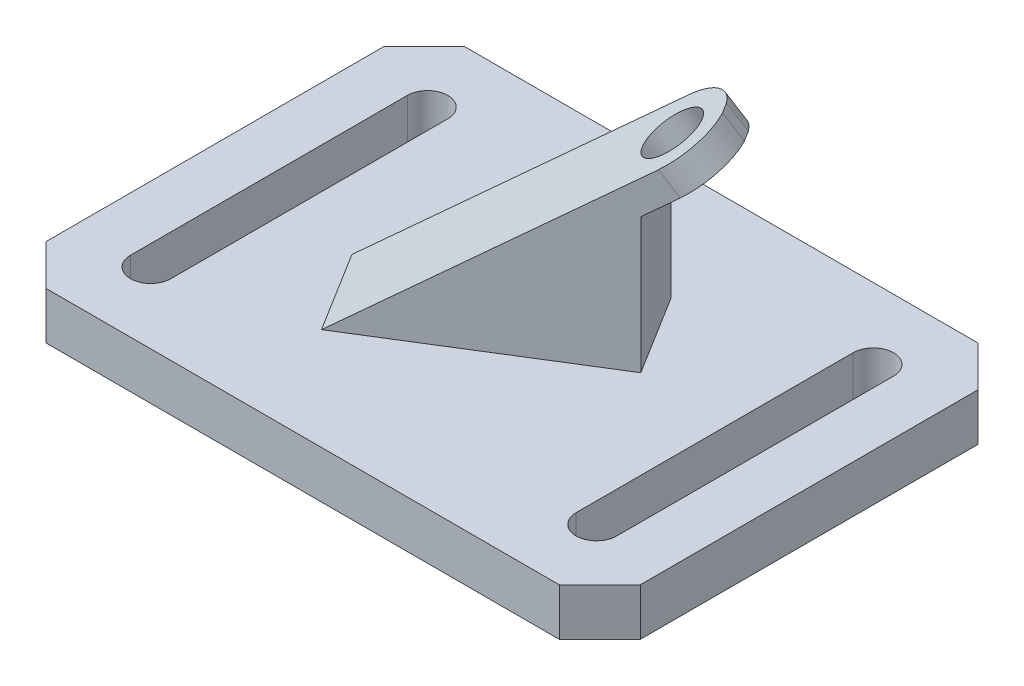
ISO-10303-21;
HEADER;
FILE_DESCRIPTION(('STEP AP214'),'2;1');
FILE_NAME('part.step','',(''),(''),'','','');
FILE_SCHEMA(('AUTOMOTIVE_DESIGN { 1 0 10303 214 1 1 1 1 }'));
ENDSEC;
DATA;
#1=APPLICATION_CONTEXT('core data for automotive mechanical design processes');
#2=APPLICATION_PROTOCOL_DEFINITION('international standard','automotive_design',2000,#1);
#3=PRODUCT_CONTEXT('',#1,'mechanical');
#4=PRODUCT('Part','Part','',(#3));
#5=PRODUCT_RELATED_PRODUCT_CATEGORY('part','',(#4));
#6=PRODUCT_DEFINITION_FORMATION('','',#4);
#7=PRODUCT_DEFINITION_CONTEXT('part definition',#1,'design');
#8=PRODUCT_DEFINITION('design','',#6,#7);
#9=PRODUCT_DEFINITION_SHAPE('','',#8);
#10=(LENGTH_UNIT() NAMED_UNIT(*) SI_UNIT(.MILLI.,.METRE.));
#11=(NAMED_UNIT(*) PLANE_ANGLE_UNIT() SI_UNIT($,.RADIAN.));
#12=(NAMED_UNIT(*) SI_UNIT($,.STERADIAN.) SOLID_ANGLE_UNIT());
#13=UNCERTAINTY_MEASURE_WITH_UNIT(LENGTH_MEASURE(1.E-05),#10,'distance_accuracy_value','');
#14=(GEOMETRIC_REPRESENTATION_CONTEXT(3) GLOBAL_UNCERTAINTY_ASSIGNED_CONTEXT((#13)) GLOBAL_UNIT_ASSIGNED_CONTEXT((#10,
#11,#12)) REPRESENTATION_CONTEXT('',''));
#15=CARTESIAN_POINT('',(0.,0.,0.));
#16=DIRECTION('',(0.,0.,1.));
#17=DIRECTION('',(1.,0.,0.));
#18=AXIS2_PLACEMENT_3D('',#15,#16,#17);
#19=CARTESIAN_POINT('',(0.,7.,0.));
#20=DIRECTION('',(0.,-1.,0.));
#21=DIRECTION('',(0.,0.,-1.));
#22=AXIS2_PLACEMENT_3D('',#19,#20,#21);
#23=PLANE('',#22);
#24=DIRECTION('',(-1.,0.,0.));
#25=VECTOR('',#24,1.);
#26=CARTESIAN_POINT('',(-44.,7.,-31.));
#27=LINE('',#26,#25);
#28=CARTESIAN_POINT('',(38.,7.,-31.));
#29=VERTEX_POINT('',#28);
#30=CARTESIAN_POINT('',(-38.,7.,-31.));
#31=VERTEX_POINT('',#30);
#32=EDGE_CURVE('E330',#29,#31,#27,.T.);
#33=ORIENTED_EDGE('',*,*,#32,.T.);
#34=DIRECTION('',(0.707106781186548,0.,-0.707106781186547));
#35=VECTOR('',#34,1.);
#36=CARTESIAN_POINT('',(-44.,7.,-25.));
#37=LINE('',#36,#35);
#38=CARTESIAN_POINT('',(-44.,7.,-25.));
#39=VERTEX_POINT('',#38);
#40=EDGE_CURVE('E372',#31,#39,#37,.F.);
#41=ORIENTED_EDGE('',*,*,#40,.T.);
#42=DIRECTION('',(0.,0.,1.));
#43=VECTOR('',#42,1.);
#44=CARTESIAN_POINT('',(-44.,7.,31.));
#45=LINE('',#44,#43);
#46=CARTESIAN_POINT('',(-44.,7.,25.));
#47=VERTEX_POINT('',#46);
#48=EDGE_CURVE('E333',#39,#47,#45,.T.);
#49=ORIENTED_EDGE('',*,*,#48,.T.);
#50=DIRECTION('',(-0.707106781186547,0.,-0.707106781186548));
#51=VECTOR('',#50,1.);
#52=CARTESIAN_POINT('',(-38.,7.,31.));
#53=LINE('',#52,#51);
#54=CARTESIAN_POINT('',(-38.,7.,31.));
#55=VERTEX_POINT('',#54);
#56=EDGE_CURVE('E368',#47,#55,#53,.F.);
#57=ORIENTED_EDGE('',*,*,#56,.T.);
#58=DIRECTION('',(1.,0.,0.));
#59=VECTOR('',#58,1.);
#60=CARTESIAN_POINT('',(-44.,7.,31.));
#61=LINE('',#60,#59);
#62=CARTESIAN_POINT('',(38.,7.,31.));
#63=VERTEX_POINT('',#62);
#64=EDGE_CURVE('E337',#55,#63,#61,.T.);
#65=ORIENTED_EDGE('',*,*,#64,.T.);
#66=DIRECTION('',(-0.707106781186548,0.,0.707106781186547));
#67=VECTOR('',#66,1.);
#68=CARTESIAN_POINT('',(44.,7.,25.));
#69=LINE('',#68,#67);
#70=CARTESIAN_POINT('',(44.,7.,25.));
#71=VERTEX_POINT('',#70);
#72=EDGE_CURVE('E369',#63,#71,#69,.F.);
#73=ORIENTED_EDGE('',*,*,#72,.T.);
#74=DIRECTION('',(0.,0.,-1.));
#75=VECTOR('',#74,1.);
#76=CARTESIAN_POINT('',(44.,7.,31.));
#77=LINE('',#76,#75);
#78=CARTESIAN_POINT('',(44.,7.,-25.));
#79=VERTEX_POINT('',#78);
#80=EDGE_CURVE('E329',#71,#79,#77,.T.);
#81=ORIENTED_EDGE('',*,*,#80,.T.);
#82=DIRECTION('',(0.707106781186547,0.,0.707106781186548));
#83=VECTOR('',#82,1.);
#84=CARTESIAN_POINT('',(38.,7.,-31.));
#85=LINE('',#84,#83);
#86=EDGE_CURVE('E375',#79,#29,#85,.F.);
#87=ORIENTED_EDGE('',*,*,#86,.T.);
#88=EDGE_LOOP('',(#33,#41,#49,#57,#65,#73,#81,#87));
#89=FACE_BOUND('',#88,.T.);
#90=DIRECTION('',(0.,0.,1.));
#91=VECTOR('',#90,1.);
#92=CARTESIAN_POINT('',(-36.,7.,-20.5));
#93=LINE('',#92,#91);
#94=CARTESIAN_POINT('',(-36.,7.,-20.5));
#95=VERTEX_POINT('',#94);
#96=CARTESIAN_POINT('',(-36.,7.,20.5));
#97=VERTEX_POINT('',#96);
#98=EDGE_CURVE('E299',#95,#97,#93,.T.);
#99=ORIENTED_EDGE('',*,*,#98,.F.);
#100=CARTESIAN_POINT('',(-33.,7.,-20.5));
#101=DIRECTION('',(0.,1.,0.));
#102=DIRECTION('',(0.,0.,1.));
#103=AXIS2_PLACEMENT_3D('',#100,#101,#102);
#104=CIRCLE('',#103,3.);
#105=CARTESIAN_POINT('',(-30.,7.,-20.5));
#106=VERTEX_POINT('',#105);
#107=EDGE_CURVE('E300',#106,#95,#104,.T.);
#108=ORIENTED_EDGE('',*,*,#107,.F.);
#109=DIRECTION('',(0.,0.,-1.));
#110=VECTOR('',#109,1.);
#111=CARTESIAN_POINT('',(-30.,7.,-20.5));
#112=LINE('',#111,#110);
#113=CARTESIAN_POINT('',(-30.,7.,20.5));
#114=VERTEX_POINT('',#113);
#115=EDGE_CURVE('E304',#114,#106,#112,.T.);
#116=ORIENTED_EDGE('',*,*,#115,.F.);
#117=CARTESIAN_POINT('',(-33.,7.,20.5));
#118=DIRECTION('',(0.,1.,0.));
#119=DIRECTION('',(0.,0.,1.));
#120=AXIS2_PLACEMENT_3D('',#117,#118,#119);
#121=CIRCLE('',#120,3.);
#122=EDGE_CURVE('E305',#97,#114,#121,.T.);
#123=ORIENTED_EDGE('',*,*,#122,.F.);
#124=EDGE_LOOP('',(#99,#108,#116,#123));
#125=FACE_BOUND('',#124,.T.);
#126=DIRECTION('',(-0.849441251034907,0.,0.527683201400473));
#127=VECTOR('',#126,1.);
#128=CARTESIAN_POINT('',(42.4093895965386,7.,-34.5859380339113));
#129=LINE('',#128,#127);
#130=CARTESIAN_POINT('',(9.45877731415572,7.,-14.116618282734));
#131=VERTEX_POINT('',#130);
#132=CARTESIAN_POINT('',(-19.7049573891051,7.,4.00024721474623));
#133=VERTEX_POINT('',#132);
#134=EDGE_CURVE('E259',#131,#133,#129,.T.);
#135=ORIENTED_EDGE('',*,*,#134,.F.);
#136=DIRECTION('',(0.527683201400473,0.,0.849441251034907));
#137=VECTOR('',#136,1.);
#138=CARTESIAN_POINT('',(-29.0620963880788,7.,-76.1258296082822));
#139=LINE('',#138,#137);
#140=CARTESIAN_POINT('',(16.8463421337624,7.,-2.22444076824528));
#141=VERTEX_POINT('',#140);
#142=EDGE_CURVE('E245',#131,#141,#139,.T.);
#143=ORIENTED_EDGE('',*,*,#142,.T.);
#144=DIRECTION('',(0.849441251034907,0.,-0.527683201400473));
#145=VECTOR('',#144,1.);
#146=CARTESIAN_POINT('',(-12.3173925694985,7.,15.892424729235));
#147=LINE('',#146,#145);
#148=CARTESIAN_POINT('',(-12.3173925694985,7.,15.892424729235));
#149=VERTEX_POINT('',#148);
#150=EDGE_CURVE('E262',#149,#141,#147,.T.);
#151=ORIENTED_EDGE('',*,*,#150,.F.);
#152=DIRECTION('',(0.527683201400473,0.,0.849441251034907));
#153=VECTOR('',#152,1.);
#154=CARTESIAN_POINT('',(-19.7049573891051,7.,4.00024721474623));
#155=LINE('',#154,#153);
#156=EDGE_CURVE('E227',#133,#149,#155,.T.);
#157=ORIENTED_EDGE('',*,*,#156,.F.);
#158=EDGE_LOOP('',(#135,#143,#151,#157));
#159=FACE_BOUND('',#158,.T.);
#160=CARTESIAN_POINT('',(33.,7.,-20.5));
#161=DIRECTION('',(0.,1.,0.));
#162=DIRECTION('',(0.,0.,1.));
#163=AXIS2_PLACEMENT_3D('',#160,#161,#162);
#164=CIRCLE('',#163,2.99999999999999);
#165=CARTESIAN_POINT('',(36.,7.,-20.5));
#166=VERTEX_POINT('',#165);
#167=CARTESIAN_POINT('',(30.,7.,-20.5));
#168=VERTEX_POINT('',#167);
#169=EDGE_CURVE('E265',#166,#168,#164,.T.);
#170=ORIENTED_EDGE('',*,*,#169,.F.);
#171=DIRECTION('',(0.,0.,-1.));
#172=VECTOR('',#171,1.);
#173=CARTESIAN_POINT('',(36.,7.,-20.5));
#174=LINE('',#173,#172);
#175=CARTESIAN_POINT('',(36.,7.,20.5));
#176=VERTEX_POINT('',#175);
#177=EDGE_CURVE('E274',#176,#166,#174,.T.);
#178=ORIENTED_EDGE('',*,*,#177,.F.);
#179=CARTESIAN_POINT('',(33.,7.,20.5));
#180=DIRECTION('',(0.,1.,0.));
#181=DIRECTION('',(0.,0.,1.));
#182=AXIS2_PLACEMENT_3D('',#179,#180,#181);
#183=CIRCLE('',#182,3.);
#184=CARTESIAN_POINT('',(30.,7.,20.5));
#185=VERTEX_POINT('',#184);
#186=EDGE_CURVE('E272',#185,#176,#183,.T.);
#187=ORIENTED_EDGE('',*,*,#186,.F.);
#188=DIRECTION('',(0.,0.,1.));
#189=VECTOR('',#188,1.);
#190=CARTESIAN_POINT('',(30.,7.,-20.5));
#191=LINE('',#190,#189);
#192=EDGE_CURVE('E268',#168,#185,#191,.T.);
#193=ORIENTED_EDGE('',*,*,#192,.F.);
#194=EDGE_LOOP('',(#170,#178,#187,#193));
#195=FACE_BOUND('',#194,.T.);
#196=ADVANCED_FACE('F41',(#89,#125,#159,#195),#23,.F.);
#197=CARTESIAN_POINT('',(0.,0.,0.));
#198=DIRECTION('',(0.,-1.,0.));
#199=DIRECTION('',(0.,0.,-1.));
#200=AXIS2_PLACEMENT_3D('',#197,#198,#199);
#201=PLANE('',#200);
#202=DIRECTION('',(0.,0.,1.));
#203=VECTOR('',#202,1.);
#204=CARTESIAN_POINT('',(-44.,0.,31.));
#205=LINE('',#204,#203);
#206=CARTESIAN_POINT('',(-44.,0.,-25.));
#207=VERTEX_POINT('',#206);
#208=CARTESIAN_POINT('',(-44.,0.,25.));
#209=VERTEX_POINT('',#208);
#210=EDGE_CURVE('E343',#207,#209,#205,.T.);
#211=ORIENTED_EDGE('',*,*,#210,.F.);
#212=DIRECTION('',(-0.707106781186548,0.,0.707106781186547));
#213=VECTOR('',#212,1.);
#214=CARTESIAN_POINT('',(-34.5,0.,-34.5));
#215=LINE('',#214,#213);
#216=CARTESIAN_POINT('',(-38.,0.,-31.));
#217=VERTEX_POINT('',#216);
#218=EDGE_CURVE('E359',#207,#217,#215,.F.);
#219=ORIENTED_EDGE('',*,*,#218,.T.);
#220=DIRECTION('',(-1.,0.,0.));
#221=VECTOR('',#220,1.);
#222=CARTESIAN_POINT('',(-44.,0.,-31.));
#223=LINE('',#222,#221);
#224=CARTESIAN_POINT('',(38.,0.,-31.));
#225=VERTEX_POINT('',#224);
#226=EDGE_CURVE('E345',#225,#217,#223,.T.);
#227=ORIENTED_EDGE('',*,*,#226,.F.);
#228=DIRECTION('',(-0.707106781186547,0.,-0.707106781186548));
#229=VECTOR('',#228,1.);
#230=CARTESIAN_POINT('',(34.5,0.,-34.5));
#231=LINE('',#230,#229);
#232=CARTESIAN_POINT('',(44.,0.,-25.));
#233=VERTEX_POINT('',#232);
#234=EDGE_CURVE('E356',#225,#233,#231,.F.);
#235=ORIENTED_EDGE('',*,*,#234,.T.);
#236=DIRECTION('',(0.,0.,-1.));
#237=VECTOR('',#236,1.);
#238=CARTESIAN_POINT('',(44.,0.,31.));
#239=LINE('',#238,#237);
#240=CARTESIAN_POINT('',(44.,0.,25.));
#241=VERTEX_POINT('',#240);
#242=EDGE_CURVE('E327',#241,#233,#239,.T.);
#243=ORIENTED_EDGE('',*,*,#242,.F.);
#244=DIRECTION('',(0.707106781186548,0.,-0.707106781186547));
#245=VECTOR('',#244,1.);
#246=CARTESIAN_POINT('',(34.5,0.,34.5));
#247=LINE('',#246,#245);
#248=CARTESIAN_POINT('',(38.,0.,31.));
#249=VERTEX_POINT('',#248);
#250=EDGE_CURVE('E358',#241,#249,#247,.F.);
#251=ORIENTED_EDGE('',*,*,#250,.T.);
#252=DIRECTION('',(1.,0.,0.));
#253=VECTOR('',#252,1.);
#254=CARTESIAN_POINT('',(-44.,0.,31.));
#255=LINE('',#254,#253);
#256=CARTESIAN_POINT('',(-38.,0.,31.));
#257=VERTEX_POINT('',#256);
#258=EDGE_CURVE('E331',#257,#249,#255,.T.);
#259=ORIENTED_EDGE('',*,*,#258,.F.);
#260=DIRECTION('',(0.707106781186547,0.,0.707106781186548));
#261=VECTOR('',#260,1.);
#262=CARTESIAN_POINT('',(-34.5,0.,34.5));
#263=LINE('',#262,#261);
#264=EDGE_CURVE('E352',#257,#209,#263,.F.);
#265=ORIENTED_EDGE('',*,*,#264,.T.);
#266=EDGE_LOOP('',(#211,#219,#227,#235,#243,#251,#259,#265));
#267=FACE_BOUND('',#266,.T.);
#268=DIRECTION('',(0.,0.,-1.));
#269=VECTOR('',#268,1.);
#270=CARTESIAN_POINT('',(-30.,0.,-20.5));
#271=LINE('',#270,#269);
#272=CARTESIAN_POINT('',(-30.,0.,20.5));
#273=VERTEX_POINT('',#272);
#274=CARTESIAN_POINT('',(-30.,0.,-20.5));
#275=VERTEX_POINT('',#274);
#276=EDGE_CURVE('E297',#273,#275,#271,.T.);
#277=ORIENTED_EDGE('',*,*,#276,.T.);
#278=CARTESIAN_POINT('',(-33.,0.,-20.5));
#279=DIRECTION('',(0.,1.,0.));
#280=DIRECTION('',(0.,0.,1.));
#281=AXIS2_PLACEMENT_3D('',#278,#279,#280);
#282=CIRCLE('',#281,3.);
#283=CARTESIAN_POINT('',(-36.,0.,-20.5));
#284=VERTEX_POINT('',#283);
#285=EDGE_CURVE('E298',#275,#284,#282,.T.);
#286=ORIENTED_EDGE('',*,*,#285,.T.);
#287=DIRECTION('',(0.,0.,1.));
#288=VECTOR('',#287,1.);
#289=CARTESIAN_POINT('',(-36.,0.,-20.5));
#290=LINE('',#289,#288);
#291=CARTESIAN_POINT('',(-36.,0.,20.5));
#292=VERTEX_POINT('',#291);
#293=EDGE_CURVE('E309',#284,#292,#290,.T.);
#294=ORIENTED_EDGE('',*,*,#293,.T.);
#295=CARTESIAN_POINT('',(-33.,0.,20.5));
#296=DIRECTION('',(0.,1.,0.));
#297=DIRECTION('',(0.,0.,1.));
#298=AXIS2_PLACEMENT_3D('',#295,#296,#297);
#299=CIRCLE('',#298,3.);
#300=EDGE_CURVE('E312',#292,#273,#299,.T.);
#301=ORIENTED_EDGE('',*,*,#300,.T.);
#302=EDGE_LOOP('',(#277,#286,#294,#301));
#303=FACE_BOUND('',#302,.T.);
#304=DIRECTION('',(0.,0.,-1.));
#305=VECTOR('',#304,1.);
#306=CARTESIAN_POINT('',(36.,0.,-20.5));
#307=LINE('',#306,#305);
#308=CARTESIAN_POINT('',(36.,0.,20.5));
#309=VERTEX_POINT('',#308);
#310=CARTESIAN_POINT('',(36.,0.,-20.5));
#311=VERTEX_POINT('',#310);
#312=EDGE_CURVE('E267',#309,#311,#307,.T.);
#313=ORIENTED_EDGE('',*,*,#312,.T.);
#314=CARTESIAN_POINT('',(33.,0.,-20.5));
#315=DIRECTION('',(0.,1.,0.));
#316=DIRECTION('',(0.,0.,1.));
#317=AXIS2_PLACEMENT_3D('',#314,#315,#316);
#318=CIRCLE('',#317,2.99999999999999);
#319=CARTESIAN_POINT('',(30.,0.,-20.5));
#320=VERTEX_POINT('',#319);
#321=EDGE_CURVE('E263',#311,#320,#318,.T.);
#322=ORIENTED_EDGE('',*,*,#321,.T.);
#323=DIRECTION('',(0.,0.,1.));
#324=VECTOR('',#323,1.);
#325=CARTESIAN_POINT('',(30.,0.,-20.5));
#326=LINE('',#325,#324);
#327=CARTESIAN_POINT('',(30.,0.,20.5));
#328=VERTEX_POINT('',#327);
#329=EDGE_CURVE('E276',#320,#328,#326,.T.);
#330=ORIENTED_EDGE('',*,*,#329,.T.);
#331=CARTESIAN_POINT('',(33.,0.,20.5));
#332=DIRECTION('',(0.,1.,0.));
#333=DIRECTION('',(0.,0.,1.));
#334=AXIS2_PLACEMENT_3D('',#331,#332,#333);
#335=CIRCLE('',#334,3.);
#336=EDGE_CURVE('E282',#328,#309,#335,.T.);
#337=ORIENTED_EDGE('',*,*,#336,.T.);
#338=EDGE_LOOP('',(#313,#322,#330,#337));
#339=FACE_BOUND('',#338,.T.);
#340=ADVANCED_FACE('F404',(#267,#303,#339),#201,.T.);
#341=CARTESIAN_POINT('',(44.,7.,31.));
#342=DIRECTION('',(-1.,0.,0.));
#343=DIRECTION('',(0.,0.,1.));
#344=AXIS2_PLACEMENT_3D('',#341,#342,#343);
#345=PLANE('',#344);
#346=ORIENTED_EDGE('',*,*,#242,.T.);
#347=DIRECTION('',(0.,1.,0.));
#348=VECTOR('',#347,1.);
#349=CARTESIAN_POINT('',(44.,7.,-25.));
#350=LINE('',#349,#348);
#351=EDGE_CURVE('E378',#233,#79,#350,.T.);
#352=ORIENTED_EDGE('',*,*,#351,.T.);
#353=ORIENTED_EDGE('',*,*,#80,.F.);
#354=DIRECTION('',(0.,-1.,0.));
#355=VECTOR('',#354,1.);
#356=CARTESIAN_POINT('',(44.,7.,25.));
#357=LINE('',#356,#355);
#358=EDGE_CURVE('E376',#71,#241,#357,.T.);
#359=ORIENTED_EDGE('',*,*,#358,.T.);
#360=EDGE_LOOP('',(#346,#352,#353,#359));
#361=FACE_BOUND('',#360,.T.);
#362=ADVANCED_FACE('F399',(#361),#345,.F.);
#363=CARTESIAN_POINT('',(-44.,7.,-31.));
#364=DIRECTION('',(0.,0.,1.));
#365=DIRECTION('',(1.,0.,0.));
#366=AXIS2_PLACEMENT_3D('',#363,#364,#365);
#367=PLANE('',#366);
#368=ORIENTED_EDGE('',*,*,#226,.T.);
#369=DIRECTION('',(0.,1.,0.));
#370=VECTOR('',#369,1.);
#371=CARTESIAN_POINT('',(-38.,7.,-31.));
#372=LINE('',#371,#370);
#373=EDGE_CURVE('E362',#217,#31,#372,.T.);
#374=ORIENTED_EDGE('',*,*,#373,.T.);
#375=ORIENTED_EDGE('',*,*,#32,.F.);
#376=DIRECTION('',(0.,-1.,0.));
#377=VECTOR('',#376,1.);
#378=CARTESIAN_POINT('',(38.,7.,-31.));
#379=LINE('',#378,#377);
#380=EDGE_CURVE('E365',#29,#225,#379,.T.);
#381=ORIENTED_EDGE('',*,*,#380,.T.);
#382=EDGE_LOOP('',(#368,#374,#375,#381));
#383=FACE_BOUND('',#382,.T.);
#384=ADVANCED_FACE('F414',(#383),#367,.F.);
#385=CARTESIAN_POINT('',(-44.,7.,31.));
#386=DIRECTION('',(1.,0.,0.));
#387=DIRECTION('',(0.,0.,-1.));
#388=AXIS2_PLACEMENT_3D('',#385,#386,#387);
#389=PLANE('',#388);
#390=ORIENTED_EDGE('',*,*,#48,.F.);
#391=DIRECTION('',(0.,-1.,0.));
#392=VECTOR('',#391,1.);
#393=CARTESIAN_POINT('',(-44.,7.,-25.));
#394=LINE('',#393,#392);
#395=EDGE_CURVE('E351',#39,#207,#394,.T.);
#396=ORIENTED_EDGE('',*,*,#395,.T.);
#397=ORIENTED_EDGE('',*,*,#210,.T.);
#398=DIRECTION('',(0.,1.,0.));
#399=VECTOR('',#398,1.);
#400=CARTESIAN_POINT('',(-44.,7.,25.));
#401=LINE('',#400,#399);
#402=EDGE_CURVE('E339',#209,#47,#401,.T.);
#403=ORIENTED_EDGE('',*,*,#402,.T.);
#404=EDGE_LOOP('',(#390,#396,#397,#403));
#405=FACE_BOUND('',#404,.T.);
#406=ADVANCED_FACE('F419',(#405),#389,.F.);
#407=CARTESIAN_POINT('',(-44.,7.,31.));
#408=DIRECTION('',(0.,0.,-1.));
#409=DIRECTION('',(-1.,0.,0.));
#410=AXIS2_PLACEMENT_3D('',#407,#408,#409);
#411=PLANE('',#410);
#412=ORIENTED_EDGE('',*,*,#258,.T.);
#413=DIRECTION('',(0.,1.,0.));
#414=VECTOR('',#413,1.);
#415=CARTESIAN_POINT('',(38.,7.,31.));
#416=LINE('',#415,#414);
#417=EDGE_CURVE('E258',#249,#63,#416,.T.);
#418=ORIENTED_EDGE('',*,*,#417,.T.);
#419=ORIENTED_EDGE('',*,*,#64,.F.);
#420=DIRECTION('',(0.,-1.,0.));
#421=VECTOR('',#420,1.);
#422=CARTESIAN_POINT('',(-38.,7.,31.));
#423=LINE('',#422,#421);
#424=EDGE_CURVE('E385',#55,#257,#423,.T.);
#425=ORIENTED_EDGE('',*,*,#424,.T.);
#426=EDGE_LOOP('',(#412,#418,#419,#425));
#427=FACE_BOUND('',#426,.T.);
#428=ADVANCED_FACE('F390',(#427),#411,.F.);
#429=CARTESIAN_POINT('',(-33.,7.,-20.5));
#430=DIRECTION('',(0.,-1.,0.));
#431=DIRECTION('',(0.,0.,-1.));
#432=AXIS2_PLACEMENT_3D('',#429,#430,#431);
#433=CYLINDRICAL_SURFACE('',#432,3.);
#434=ORIENTED_EDGE('',*,*,#285,.F.);
#435=DIRECTION('',(0.,-1.,0.));
#436=VECTOR('',#435,1.);
#437=CARTESIAN_POINT('',(-30.,7.,-20.5));
#438=LINE('',#437,#436);
#439=EDGE_CURVE('E310',#106,#275,#438,.T.);
#440=ORIENTED_EDGE('',*,*,#439,.F.);
#441=ORIENTED_EDGE('',*,*,#107,.T.);
#442=DIRECTION('',(0.,-1.,0.));
#443=VECTOR('',#442,1.);
#444=CARTESIAN_POINT('',(-36.,7.,-20.5));
#445=LINE('',#444,#443);
#446=EDGE_CURVE('E321',#95,#284,#445,.T.);
#447=ORIENTED_EDGE('',*,*,#446,.T.);
#448=EDGE_LOOP('',(#434,#440,#441,#447));
#449=FACE_BOUND('',#448,.T.);
#450=ADVANCED_FACE('F437',(#449),#433,.F.);
#451=CARTESIAN_POINT('',(-36.,7.,-20.5));
#452=DIRECTION('',(1.,0.,0.));
#453=DIRECTION('',(0.,0.,-1.));
#454=AXIS2_PLACEMENT_3D('',#451,#452,#453);
#455=PLANE('',#454);
#456=ORIENTED_EDGE('',*,*,#293,.F.);
#457=ORIENTED_EDGE('',*,*,#446,.F.);
#458=ORIENTED_EDGE('',*,*,#98,.T.);
#459=DIRECTION('',(0.,-1.,0.));
#460=VECTOR('',#459,1.);
#461=CARTESIAN_POINT('',(-36.,7.,20.5));
#462=LINE('',#461,#460);
#463=EDGE_CURVE('E325',#97,#292,#462,.T.);
#464=ORIENTED_EDGE('',*,*,#463,.T.);
#465=EDGE_LOOP('',(#456,#457,#458,#464));
#466=FACE_BOUND('',#465,.T.);
#467=ADVANCED_FACE('F635',(#466),#455,.T.);
#468=CARTESIAN_POINT('',(-33.,7.,20.5));
#469=DIRECTION('',(0.,-1.,0.));
#470=DIRECTION('',(0.,0.,-1.));
#471=AXIS2_PLACEMENT_3D('',#468,#469,#470);
#472=CYLINDRICAL_SURFACE('',#471,3.);
#473=ORIENTED_EDGE('',*,*,#300,.F.);
#474=ORIENTED_EDGE('',*,*,#463,.F.);
#475=ORIENTED_EDGE('',*,*,#122,.T.);
#476=DIRECTION('',(0.,-1.,0.));
#477=VECTOR('',#476,1.);
#478=CARTESIAN_POINT('',(-30.,7.,20.5));
#479=LINE('',#478,#477);
#480=EDGE_CURVE('E318',#114,#273,#479,.T.);
#481=ORIENTED_EDGE('',*,*,#480,.T.);
#482=EDGE_LOOP('',(#473,#474,#475,#481));
#483=FACE_BOUND('',#482,.T.);
#484=ADVANCED_FACE('F621',(#483),#472,.F.);
#485=CARTESIAN_POINT('',(-30.,7.,-20.5));
#486=DIRECTION('',(-1.,0.,0.));
#487=DIRECTION('',(0.,0.,1.));
#488=AXIS2_PLACEMENT_3D('',#485,#486,#487);
#489=PLANE('',#488);
#490=ORIENTED_EDGE('',*,*,#276,.F.);
#491=ORIENTED_EDGE('',*,*,#480,.F.);
#492=ORIENTED_EDGE('',*,*,#115,.T.);
#493=ORIENTED_EDGE('',*,*,#439,.T.);
#494=EDGE_LOOP('',(#490,#491,#492,#493));
#495=FACE_BOUND('',#494,.T.);
#496=ADVANCED_FACE('F612',(#495),#489,.T.);
#497=CARTESIAN_POINT('',(33.,7.,-20.5));
#498=DIRECTION('',(0.,-1.,0.));
#499=DIRECTION('',(0.,0.,-1.));
#500=AXIS2_PLACEMENT_3D('',#497,#498,#499);
#501=CYLINDRICAL_SURFACE('',#500,2.99999999999999);
#502=ORIENTED_EDGE('',*,*,#321,.F.);
#503=DIRECTION('',(0.,-1.,0.));
#504=VECTOR('',#503,1.);
#505=CARTESIAN_POINT('',(36.,7.,-20.5));
#506=LINE('',#505,#504);
#507=EDGE_CURVE('E277',#166,#311,#506,.T.);
#508=ORIENTED_EDGE('',*,*,#507,.F.);
#509=ORIENTED_EDGE('',*,*,#169,.T.);
#510=DIRECTION('',(0.,-1.,0.));
#511=VECTOR('',#510,1.);
#512=CARTESIAN_POINT('',(30.,7.,-20.5));
#513=LINE('',#512,#511);
#514=EDGE_CURVE('E291',#168,#320,#513,.T.);
#515=ORIENTED_EDGE('',*,*,#514,.T.);
#516=EDGE_LOOP('',(#502,#508,#509,#515));
#517=FACE_BOUND('',#516,.T.);
#518=ADVANCED_FACE('F603',(#517),#501,.F.);
#519=CARTESIAN_POINT('',(30.,7.,-20.5));
#520=DIRECTION('',(1.,0.,0.));
#521=DIRECTION('',(0.,0.,-1.));
#522=AXIS2_PLACEMENT_3D('',#519,#520,#521);
#523=PLANE('',#522);
#524=ORIENTED_EDGE('',*,*,#329,.F.);
#525=ORIENTED_EDGE('',*,*,#514,.F.);
#526=ORIENTED_EDGE('',*,*,#192,.T.);
#527=DIRECTION('',(0.,-1.,0.));
#528=VECTOR('',#527,1.);
#529=CARTESIAN_POINT('',(30.,7.,20.5));
#530=LINE('',#529,#528);
#531=EDGE_CURVE('E293',#185,#328,#530,.T.);
#532=ORIENTED_EDGE('',*,*,#531,.T.);
#533=EDGE_LOOP('',(#524,#525,#526,#532));
#534=FACE_BOUND('',#533,.T.);
#535=ADVANCED_FACE('F597',(#534),#523,.T.);
#536=CARTESIAN_POINT('',(33.,7.,20.5));
#537=DIRECTION('',(0.,-1.,0.));
#538=DIRECTION('',(0.,0.,-1.));
#539=AXIS2_PLACEMENT_3D('',#536,#537,#538);
#540=CYLINDRICAL_SURFACE('',#539,3.);
#541=ORIENTED_EDGE('',*,*,#336,.F.);
#542=ORIENTED_EDGE('',*,*,#531,.F.);
#543=ORIENTED_EDGE('',*,*,#186,.T.);
#544=DIRECTION('',(0.,-1.,0.));
#545=VECTOR('',#544,1.);
#546=CARTESIAN_POINT('',(36.,7.,20.5));
#547=LINE('',#546,#545);
#548=EDGE_CURVE('E287',#176,#309,#547,.T.);
#549=ORIENTED_EDGE('',*,*,#548,.T.);
#550=EDGE_LOOP('',(#541,#542,#543,#549));
#551=FACE_BOUND('',#550,.T.);
#552=ADVANCED_FACE('F587',(#551),#540,.F.);
#553=CARTESIAN_POINT('',(36.,7.,-20.5));
#554=DIRECTION('',(-1.,0.,0.));
#555=DIRECTION('',(0.,0.,1.));
#556=AXIS2_PLACEMENT_3D('',#553,#554,#555);
#557=PLANE('',#556);
#558=ORIENTED_EDGE('',*,*,#312,.F.);
#559=ORIENTED_EDGE('',*,*,#548,.F.);
#560=ORIENTED_EDGE('',*,*,#177,.T.);
#561=ORIENTED_EDGE('',*,*,#507,.T.);
#562=EDGE_LOOP('',(#558,#559,#560,#561));
#563=FACE_BOUND('',#562,.T.);
#564=ADVANCED_FACE('F453',(#563),#557,.T.);
#565=CARTESIAN_POINT('',(-44.,7.,-25.));
#566=DIRECTION('',(0.707106781186547,0.,0.707106781186548));
#567=DIRECTION('',(0.,-1.,0.));
#568=AXIS2_PLACEMENT_3D('',#565,#566,#567);
#569=PLANE('',#568);
#570=ORIENTED_EDGE('',*,*,#40,.F.);
#571=ORIENTED_EDGE('',*,*,#373,.F.);
#572=ORIENTED_EDGE('',*,*,#218,.F.);
#573=ORIENTED_EDGE('',*,*,#395,.F.);
#574=EDGE_LOOP('',(#570,#571,#572,#573));
#575=FACE_BOUND('',#574,.T.);
#576=ADVANCED_FACE('F422',(#575),#569,.F.);
#577=CARTESIAN_POINT('',(38.,7.,-31.));
#578=DIRECTION('',(-0.707106781186548,0.,0.707106781186547));
#579=DIRECTION('',(0.,-1.,0.));
#580=AXIS2_PLACEMENT_3D('',#577,#578,#579);
#581=PLANE('',#580);
#582=ORIENTED_EDGE('',*,*,#86,.F.);
#583=ORIENTED_EDGE('',*,*,#351,.F.);
#584=ORIENTED_EDGE('',*,*,#234,.F.);
#585=ORIENTED_EDGE('',*,*,#380,.F.);
#586=EDGE_LOOP('',(#582,#583,#584,#585));
#587=FACE_BOUND('',#586,.T.);
#588=ADVANCED_FACE('F408',(#587),#581,.F.);
#589=CARTESIAN_POINT('',(44.,7.,25.));
#590=DIRECTION('',(-0.707106781186547,0.,-0.707106781186548));
#591=DIRECTION('',(0.,-1.,0.));
#592=AXIS2_PLACEMENT_3D('',#589,#590,#591);
#593=PLANE('',#592);
#594=ORIENTED_EDGE('',*,*,#72,.F.);
#595=ORIENTED_EDGE('',*,*,#417,.F.);
#596=ORIENTED_EDGE('',*,*,#250,.F.);
#597=ORIENTED_EDGE('',*,*,#358,.F.);
#598=EDGE_LOOP('',(#594,#595,#596,#597));
#599=FACE_BOUND('',#598,.T.);
#600=ADVANCED_FACE('F400',(#599),#593,.F.);
#601=CARTESIAN_POINT('',(-38.,7.,31.));
#602=DIRECTION('',(0.707106781186548,0.,-0.707106781186547));
#603=DIRECTION('',(0.,-1.,0.));
#604=AXIS2_PLACEMENT_3D('',#601,#602,#603);
#605=PLANE('',#604);
#606=ORIENTED_EDGE('',*,*,#56,.F.);
#607=ORIENTED_EDGE('',*,*,#402,.F.);
#608=ORIENTED_EDGE('',*,*,#264,.F.);
#609=ORIENTED_EDGE('',*,*,#424,.F.);
#610=EDGE_LOOP('',(#606,#607,#608,#609));
#611=FACE_BOUND('',#610,.T.);
#612=ADVANCED_FACE('F42',(#611),#605,.F.);
#613=CARTESIAN_POINT('',(42.4093895965386,94.,-34.5859380339113));
#614=DIRECTION('',(0.527683201400473,0.,0.849441251034907));
#615=DIRECTION('',(0.849441251034907,0.,-0.527683201400473));
#616=AXIS2_PLACEMENT_3D('',#613,#614,#615);
#617=PLANE('',#616);
#618=DIRECTION('',(0.687212407810358,0.587785252292469,-0.426904677579163));
#619=VECTOR('',#618,1.);
#620=CARTESIAN_POINT('',(56.0916092200396,71.8301798991289,-43.0854987091165));
#621=LINE('',#620,#619);
#622=CARTESIAN_POINT('',(11.3603506914492,33.5707221524889,-15.297898714083));
#623=VERTEX_POINT('',#622);
#624=EDGE_CURVE('E63',#133,#623,#621,.T.);
#625=ORIENTED_EDGE('',*,*,#624,.T.);
#626=DIRECTION('',(-0.499289040047183,0.80901699437495,0.310164403665675));
#627=VECTOR('',#626,1.);
#628=CARTESIAN_POINT('',(14.8553739717795,27.9076031918642,-17.4690495397427));
#629=LINE('',#628,#627);
#630=CARTESIAN_POINT('',(13.357506851638,30.3346541749891,-16.5385563287457));
#631=VERTEX_POINT('',#630);
#632=EDGE_CURVE('E718',#623,#631,#629,.F.);
#633=ORIENTED_EDGE('',*,*,#632,.T.);
#634=DIRECTION('',(-0.687212407810357,-0.58778525229247,0.426904677579162));
#635=VECTOR('',#634,1.);
#636=CARTESIAN_POINT('',(58.0887653802283,68.5941119216292,-44.3261563237791));
#637=LINE('',#636,#635);
#638=CARTESIAN_POINT('',(9.45877731415571,27.,-14.116618282734));
#639=VERTEX_POINT('',#638);
#640=EDGE_CURVE('E254',#631,#639,#637,.T.);
#641=ORIENTED_EDGE('',*,*,#640,.T.);
#642=DIRECTION('',(0.,-1.,0.));
#643=VECTOR('',#642,1.);
#644=CARTESIAN_POINT('',(9.4587773141557,94.,-14.116618282734));
#645=LINE('',#644,#643);
#646=EDGE_CURVE('E253',#639,#131,#645,.T.);
#647=ORIENTED_EDGE('',*,*,#646,.T.);
#648=ORIENTED_EDGE('',*,*,#134,.T.);
#649=EDGE_LOOP('',(#625,#633,#641,#647,#648));
#650=FACE_BOUND('',#649,.T.);
#651=ADVANCED_FACE('F424',(#650),#617,.F.);
#652=CARTESIAN_POINT('',(-12.3173925694985,94.,15.892424729235));
#653=DIRECTION('',(-0.527683201400473,0.,-0.849441251034907));
#654=DIRECTION('',(-0.849441251034907,0.,0.527683201400473));
#655=AXIS2_PLACEMENT_3D('',#652,#653,#654);
#656=PLANE('',#655);
#657=DIRECTION('',(-0.687212407810358,-0.58778525229247,0.426904677579162));
#658=VECTOR('',#657,1.);
#659=CARTESIAN_POINT('',(25.0928910274866,34.0534230275096,-7.3472968991952));
#660=LINE('',#659,#658);
#661=CARTESIAN_POINT('',(20.4472132904088,30.0798904927022,-4.46134557767718));
#662=VERTEX_POINT('',#661);
#663=CARTESIAN_POINT('',(16.8463421337624,27.,-2.22444076824528));
#664=VERTEX_POINT('',#663);
#665=EDGE_CURVE('E220',#662,#664,#660,.T.);
#666=ORIENTED_EDGE('',*,*,#665,.F.);
#667=DIRECTION('',(-0.499289040047184,0.80901699437495,0.310164403665675));
#668=VECTOR('',#667,1.);
#669=CARTESIAN_POINT('',(-16.6921415795693,90.2581977255127,18.6100718415517));
#670=LINE('',#669,#668);
#671=CARTESIAN_POINT('',(18.4500571302201,33.3159584702021,-3.22068796301451));
#672=VERTEX_POINT('',#671);
#673=EDGE_CURVE('E204',#662,#672,#670,.T.);
#674=ORIENTED_EDGE('',*,*,#673,.T.);
#675=DIRECTION('',(0.687212407810358,0.587785252292469,-0.426904677579162));
#676=VECTOR('',#675,1.);
#677=CARTESIAN_POINT('',(-12.3173925694985,7.,15.892424729235));
#678=LINE('',#677,#676);
#679=EDGE_CURVE('E217',#149,#672,#678,.T.);
#680=ORIENTED_EDGE('',*,*,#679,.F.);
#681=ORIENTED_EDGE('',*,*,#150,.T.);
#682=DIRECTION('',(0.,-1.,0.));
#683=VECTOR('',#682,1.);
#684=CARTESIAN_POINT('',(16.8463421337624,27.,-2.22444076824528));
#685=LINE('',#684,#683);
#686=EDGE_CURVE('E229',#664,#141,#685,.T.);
#687=ORIENTED_EDGE('',*,*,#686,.F.);
#688=EDGE_LOOP('',(#666,#674,#680,#681,#687));
#689=FACE_BOUND('',#688,.T.);
#690=ADVANCED_FACE('F213',(#689),#656,.F.);
#691=CARTESIAN_POINT('',(-29.0620963880788,27.,-76.1258296082822));
#692=DIRECTION('',(-0.849441251034907,0.,0.527683201400473));
#693=DIRECTION('',(0.527683201400473,0.,0.849441251034907));
#694=AXIS2_PLACEMENT_3D('',#691,#692,#693);
#695=PLANE('',#694);
#696=DIRECTION('',(0.527683201400473,0.,0.849441251034907));
#697=VECTOR('',#696,1.);
#698=CARTESIAN_POINT('',(-29.0620963880788,27.,-76.1258296082822));
#699=LINE('',#698,#697);
#700=EDGE_CURVE('E242',#639,#664,#699,.T.);
#701=ORIENTED_EDGE('',*,*,#700,.T.);
#702=ORIENTED_EDGE('',*,*,#686,.T.);
#703=ORIENTED_EDGE('',*,*,#142,.F.);
#704=ORIENTED_EDGE('',*,*,#646,.F.);
#705=EDGE_LOOP('',(#701,#702,#703,#704));
#706=FACE_BOUND('',#705,.T.);
#707=ADVANCED_FACE('F471',(#706),#695,.F.);
#708=CARTESIAN_POINT('',(-20.8155474943545,34.0534230275096,-81.2486857392321));
#709=DIRECTION('',(-0.499289040047184,0.80901699437495,0.310164403665675));
#710=DIRECTION('',(-0.850985081019818,-0.525189862698905,0.));
#711=AXIS2_PLACEMENT_3D('',#708,#709,#710);
#712=PLANE('',#711);
#713=CARTESIAN_POINT('',(16.6153438131044,29.973946318314,-10.3533814585714));
#714=DIRECTION('',(-0.499289040047184,0.80901699437495,0.310164403665675));
#715=DIRECTION('',(-0.850985081019818,-0.525189862698905,0.));
#716=AXIS2_PLACEMENT_3D('',#713,#714,#715);
#717=CIRCLE('',#716,4.);
#718=CARTESIAN_POINT('',(13.2114034890251,27.8731868675183,-10.3533814585714));
#719=VERTEX_POINT('',#718);
#720=EDGE_CURVE('E208',#719,#719,#717,.T.);
#721=ORIENTED_EDGE('',*,*,#720,.T.);
#722=EDGE_LOOP('',(#721));
#723=FACE_BOUND('',#722,.T.);
#724=ORIENTED_EDGE('',*,*,#640,.F.);
#725=CARTESIAN_POINT('',(16.6153438131044,29.9739463183139,-10.3533814585714));
#726=DIRECTION('',(-0.499289040047184,0.80901699437495,0.310164403665675));
#727=DIRECTION('',(-0.850985081019818,-0.525189862698905,0.));
#728=AXIS2_PLACEMENT_3D('',#725,#726,#727);
#729=CIRCLE('',#728,7.);
#730=CARTESIAN_POINT('',(20.9039806752057,34.0534230275096,-14.0904208809157));
#731=VERTEX_POINT('',#730);
#732=EDGE_CURVE('E232',#631,#731,#729,.F.);
#733=ORIENTED_EDGE('',*,*,#732,.T.);
#734=DIRECTION('',(0.527683201400473,0.,0.849441251034907));
#735=VECTOR('',#734,1.);
#736=CARTESIAN_POINT('',(-20.8155474943545,34.0534230275096,-81.2486857392321));
#737=LINE('',#736,#735);
#738=CARTESIAN_POINT('',(21.8657928705582,34.0534230275096,-12.5421378347386));
#739=VERTEX_POINT('',#738);
#740=EDGE_CURVE('E250',#731,#739,#737,.T.);
#741=ORIENTED_EDGE('',*,*,#740,.T.);
#742=CARTESIAN_POINT('',(20.3450511211873,30.004762147567,-4.42984081291864));
#743=VERTEX_POINT('',#742);
#744=EDGE_CURVE('E226',#739,#743,#729,.F.);
#745=ORIENTED_EDGE('',*,*,#744,.T.);
#746=DIRECTION('',(0.781849913187288,0.574959308024922,-0.241106838070869));
#747=VECTOR('',#746,1.);
#748=CARTESIAN_POINT('',(11.4850916334468,23.4892965955744,-1.69760693849548));
#749=LINE('',#748,#747);
#750=EDGE_CURVE('E225',#743,#662,#749,.T.);
#751=ORIENTED_EDGE('',*,*,#750,.T.);
#752=ORIENTED_EDGE('',*,*,#665,.T.);
#753=ORIENTED_EDGE('',*,*,#700,.F.);
#754=EDGE_LOOP('',(#724,#733,#741,#745,#751,#752,#753));
#755=FACE_BOUND('',#754,.T.);
#756=ADVANCED_FACE('F477',(#723,#755),#712,.F.);
#757=CARTESIAN_POINT('',(-22.8127036545432,37.2894910050094,-80.0080281245694));
#758=DIRECTION('',(-0.687212407810358,-0.587785252292469,0.426904677579162));
#759=DIRECTION('',(0.649991642509844,-0.759941356071214,0.));
#760=AXIS2_PLACEMENT_3D('',#757,#758,#759);
#761=PLANE('',#760);
#762=DIRECTION('',(0.527683201400473,0.,0.849441251034907));
#763=VECTOR('',#762,1.);
#764=CARTESIAN_POINT('',(-22.8127036545432,37.2894910050094,-80.0080281245694));
#765=LINE('',#764,#763);
#766=CARTESIAN_POINT('',(18.906824515017,37.2894910050094,-12.849763266253));
#767=VERTEX_POINT('',#766);
#768=CARTESIAN_POINT('',(19.8686367103694,37.2894910050094,-11.3014802200759));
#769=VERTEX_POINT('',#768);
#770=EDGE_CURVE('E241',#767,#769,#765,.T.);
#771=ORIENTED_EDGE('',*,*,#770,.T.);
#772=DIRECTION('',(-0.499289040047183,0.80901699437495,0.310164403665675));
#773=VECTOR('',#772,1.);
#774=CARTESIAN_POINT('',(23.3636599906997,31.6263720443848,-13.4726310457356));
#775=LINE('',#774,#773);
#776=EDGE_CURVE('E231',#769,#739,#775,.F.);
#777=ORIENTED_EDGE('',*,*,#776,.T.);
#778=ORIENTED_EDGE('',*,*,#740,.F.);
#779=DIRECTION('',(-0.499289040047183,0.80901699437495,0.310164403665675));
#780=VECTOR('',#779,1.);
#781=CARTESIAN_POINT('',(22.4018477953472,31.6263720443848,-15.0209140919127));
#782=LINE('',#781,#780);
#783=EDGE_CURVE('E221',#731,#767,#782,.T.);
#784=ORIENTED_EDGE('',*,*,#783,.T.);
#785=EDGE_LOOP('',(#771,#777,#778,#784));
#786=FACE_BOUND('',#785,.T.);
#787=ADVANCED_FACE('F498',(#786),#761,.F.);
#788=CARTESIAN_POINT('',(-58.2258310913396,7.,-58.0089641108019));
#789=DIRECTION('',(0.499289040047183,-0.809016994374951,-0.310164403665675));
#790=DIRECTION('',(0.850985081019819,0.525189862698903,0.));
#791=AXIS2_PLACEMENT_3D('',#788,#789,#790);
#792=PLANE('',#791);
#793=CARTESIAN_POINT('',(14.6181876529156,33.2100142958138,-9.11272384390868));
#794=DIRECTION('',(-0.499289040047183,0.809016994374951,0.310164403665675));
#795=DIRECTION('',(-0.850985081019819,-0.525189862698903,0.));
#796=AXIS2_PLACEMENT_3D('',#793,#794,#795);
#797=CIRCLE('',#796,4.);
#798=CARTESIAN_POINT('',(11.2142473288364,31.1092548450182,-9.11272384390868));
#799=VERTEX_POINT('',#798);
#800=EDGE_CURVE('E724',#799,#799,#797,.T.);
#801=ORIENTED_EDGE('',*,*,#800,.F.);
#802=EDGE_LOOP('',(#801));
#803=FACE_BOUND('',#802,.T.);
#804=ORIENTED_EDGE('',*,*,#770,.F.);
#805=CARTESIAN_POINT('',(14.6181876529156,33.2100142958138,-9.11272384390868));
#806=DIRECTION('',(0.499289040047183,-0.809016994374951,-0.310164403665675));
#807=DIRECTION('',(0.850985081019819,0.525189862698903,0.));
#808=AXIS2_PLACEMENT_3D('',#805,#806,#807);
#809=CIRCLE('',#808,7.);
#810=EDGE_CURVE('E11',#767,#623,#809,.F.);
#811=ORIENTED_EDGE('',*,*,#810,.T.);
#812=ORIENTED_EDGE('',*,*,#624,.F.);
#813=ORIENTED_EDGE('',*,*,#156,.T.);
#814=ORIENTED_EDGE('',*,*,#679,.T.);
#815=DIRECTION('',(0.78184991318729,0.57495930802492,-0.241106838070869));
#816=VECTOR('',#815,1.);
#817=CARTESIAN_POINT('',(22.0853751001635,35.9893103107471,-4.34174714116562));
#818=LINE('',#817,#816);
#819=CARTESIAN_POINT('',(18.3478949609986,33.2408301250668,-3.18918319825594));
#820=VERTEX_POINT('',#819);
#821=EDGE_CURVE('E205',#820,#672,#818,.T.);
#822=ORIENTED_EDGE('',*,*,#821,.F.);
#823=EDGE_CURVE('E46',#820,#769,#809,.F.);
#824=ORIENTED_EDGE('',*,*,#823,.T.);
#825=EDGE_LOOP('',(#804,#811,#812,#813,#814,#822,#824));
#826=FACE_BOUND('',#825,.T.);
#827=ADVANCED_FACE('F224',(#803,#826),#792,.F.);
#828=CARTESIAN_POINT('',(25.5803983804938,30.3261913501225,-6.51289796682534));
#829=DIRECTION('',(0.373391440364921,-0.122120010350579,0.919600747789052));
#830=DIRECTION('',(0.926535549987906,0.,-0.376207222961772));
#831=AXIS2_PLACEMENT_3D('',#828,#829,#830);
#832=PLANE('',#831);
#833=ORIENTED_EDGE('',*,*,#750,.F.);
#834=DIRECTION('',(-0.499289040047183,0.80901699437495,0.310164403665675));
#835=VECTOR('',#834,1.);
#836=CARTESIAN_POINT('',(21.8429182413289,27.5777111644421,-5.36033402391567));
#837=LINE('',#836,#835);
#838=EDGE_CURVE('E60',#743,#820,#837,.T.);
#839=ORIENTED_EDGE('',*,*,#838,.T.);
#840=ORIENTED_EDGE('',*,*,#821,.T.);
#841=ORIENTED_EDGE('',*,*,#673,.F.);
#842=EDGE_LOOP('',(#833,#839,#840,#841));
#843=FACE_BOUND('',#842,.T.);
#844=ADVANCED_FACE('F202',(#843),#832,.F.);
#845=CARTESIAN_POINT('',(18.1132109332459,27.5468953351891,-11.2838746695684));
#846=DIRECTION('',(-0.499289040047183,0.80901699437495,0.310164403665675));
#847=DIRECTION('',(-0.850985081019819,-0.525189862698903,0.));
#848=AXIS2_PLACEMENT_3D('',#845,#846,#847);
#849=CYLINDRICAL_SURFACE('',#848,7.);
#850=ORIENTED_EDGE('',*,*,#776,.F.);
#851=ORIENTED_EDGE('',*,*,#823,.F.);
#852=ORIENTED_EDGE('',*,*,#838,.F.);
#853=ORIENTED_EDGE('',*,*,#744,.F.);
#854=EDGE_LOOP('',(#850,#851,#852,#853));
#855=FACE_BOUND('',#854,.T.);
#856=ADVANCED_FACE('F512',(#855),#849,.T.);
#857=ORIENTED_EDGE('',*,*,#810,.F.);
#858=ORIENTED_EDGE('',*,*,#783,.F.);
#859=ORIENTED_EDGE('',*,*,#732,.F.);
#860=ORIENTED_EDGE('',*,*,#632,.F.);
#861=EDGE_LOOP('',(#857,#858,#859,#860));
#862=FACE_BOUND('',#861,.T.);
#863=ADVANCED_FACE('F516',(#862),#849,.T.);
#864=CARTESIAN_POINT('',(23.1061013337177,19.4567253914396,-14.3855187062252));
#865=DIRECTION('',(-0.499289040047183,0.80901699437495,0.310164403665675));
#866=DIRECTION('',(-0.850985081019819,-0.525189862698903,0.));
#867=AXIS2_PLACEMENT_3D('',#864,#865,#866);
#868=CYLINDRICAL_SURFACE('',#867,4.);
#869=ORIENTED_EDGE('',*,*,#800,.T.);
#870=EDGE_LOOP('',(#869));
#871=FACE_BOUND('',#870,.T.);
#872=ORIENTED_EDGE('',*,*,#720,.F.);
#873=EDGE_LOOP('',(#872));
#874=FACE_BOUND('',#873,.T.);
#875=ADVANCED_FACE('F528',(#871,#874),#868,.F.);
#876=CLOSED_SHELL('',(#196,#340,#362,#384,#406,#428,#450,#467,#484,#496,#518,#535,#552,#564,
#576,#588,#600,#612,#651,#690,#707,#756,#787,#827,#844,#856,#863,#875));
#877=MANIFOLD_SOLID_BREP('B2',#876);
#878=ADVANCED_BREP_SHAPE_REPRESENTATION('',(#18,#877),#14);
#879=SHAPE_DEFINITION_REPRESENTATION(#9,#878);
ENDSEC;
END-ISO-10303-21;
